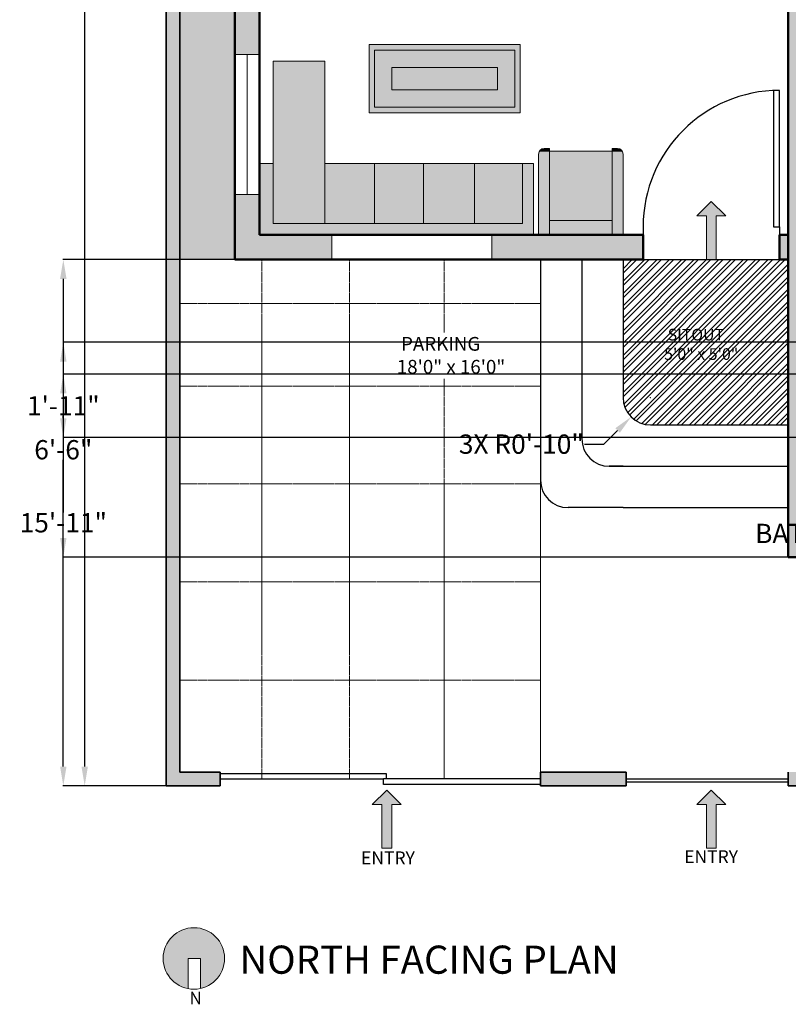
# Model space of a CAD drawing. Units: inches. Extents: x 319 to 870, y 210 to 995.
# Tile 1 of 6: x 319 to 598, y 245 to 603. Entities that reach past the tile are written whole.
import ezdxf

# ---------------------------------------------------------------- set-up
doc = ezdxf.new("R2010")
doc.units = ezdxf.units.IN
doc.header["$MEASUREMENT"] = 0
doc.linetypes.add('DASHED2', pattern=[0.375, 0.25, -0.125])
for name, color, linetype, lineweight in [('A-ANNO-DIMS', 2, 'Continuous', 18), ('A-ANNO-SYMB', 7, 'Continuous', 18), ('A-ANNO-TEXT', 7, 'Continuous', 18), ('A-ANNO-TITL', 7, 'Continuous', 35), ('A-AREA-IDEN', 7, 'Continuous', 18), ('A-DOOR', 4, 'Continuous', 25), ('A-FLOR-PATT', 252, 'Continuous', 13), ('A-FLOR-STRS', 7, 'Continuous', 25), ('A-FURN', 8, 'Continuous', 18), ('A-GLAZ', 4, 'Continuous', 18), ('A-WALL', 7, 'Continuous', 50), ('A-WALL-PATT', 8, 'Continuous', 13), ('C-PROP', 7, 'Continuous', 35), ('C-PROP-PATT', 8, 'Continuous', 13), ('C-PVMT-JNTS', 8, 'DASHED2', 13), ('C-SITE-GATE', 4, 'Continuous', 25)]:
    doc.layers.add(name, color=color, linetype=linetype, lineweight=lineweight)
for name, color, linetype, lineweight, true_color in [('A-ANNO-SYMB-PATT', 16, 'Continuous', 13, 0x6c0707), ('A-FURN-PATT', 30, 'Continuous', 13, 0xf7941d), ('C-SITE-PATT', 126, 'Continuous', 13, 0x1e6f63)]:
    doc.layers.add(name, color=color, linetype=linetype, lineweight=lineweight, true_color=true_color)
doc.styles.get("Standard").update_dxf_attribs({"font": 'arial.ttf'})
doc.dimstyles.get("Standard").update_dxf_attribs({"dimtxt": 7, "dimasz": 7, "dimexe": 0.18, "dimexo": 0.0625, "dimgap": 0.09, "dimtad": 0, "dimtih": 1, "dimtoh": 1, "dimdec": 0, "dimzin": 0, "dimdsep": 46, "dimlunit": 3, "dimtxsty": 'Standard', "dimcen": 0.09, "dimadec": 0, "dimazin": 0, "dimtfac": 1, "dimtdec": 0, "dimtofl": 0, "dimtmove": 0, "dimatfit": 3, "dimfxl": 1, "dimtolj": 1, "dimtzin": 0, "dimarcsym": 0})

# ---------------------------------------------------------------- blocks, each defined once
blk = doc.blocks.new('*U12')
for p, q in [((0, 0), (0, -6)), ((-40, 0), (-40, -6))]:
    blk.add_line(p, q)
blk.add_lwpolyline([(0, 0), (0, 40), (-1.75, 40), (-1.75, 0)], close=True)
blk.add_arc((0, 0), 40, 90, 180)
blk = doc.blocks.new('Arrows - Metric')
h = blk.add_hatch(color=0)
h.set_gradient(color1=(0, 0, 255), rotation=180, tint=1)
h.paths.add_polyline_path([(0, 0), (-6.35, -6.35), (-6.35, -2.159), (-25.4, -2.159), (-25.4, 2.159), (-6.35, 2.159), (-6.35, 6.35)])
at = {"color": 0}
blk.add_lwpolyline([(0, 0), (-6.35, -6.35), (-6.35, -2.159), (-25.4, -2.159), (-25.4, 2.159), (-6.35, 2.159), (-6.35, 6.35)], close=True, dxfattribs=at)
blk = doc.blocks.new('*D22')
at = {"layer": 'A-ANNO-DIMS', "color": 0, "lineweight": -2, "transparency": 16777216}
for p, q in [((371.62, 948.67), (341.96, 948.67)), ((342.14, 941.67), (342.14, 640.33)), ((342.14, 331.67), (342.14, 633)), ((371.62, 324.67), (341.96, 324.67))]:
    blk.add_line(p, q, dxfattribs=at)
at = {"layer": 'A-ANNO-DIMS', "color": 0, "transparency": 16777216}
for points in [[(340.97, 941.67), (343.31, 941.67), (342.14, 948.67)], [(340.97, 331.67), (343.31, 331.67), (342.14, 324.67)]]:
    blk.add_solid(points, dxfattribs=at)
at = {"layer": 'Defpoints', "color": 0, "transparency": 16777216}
for p in [(371.68, 948.67), (342.14, 324.67), (371.68, 324.67)]:
    blk.add_point(p, dxfattribs=at)
at = {"layer": 'A-ANNO-DIMS', "color": 0, "transparency": 16777216, "insert": (342.14, 636.67), "char_height": 7, "attachment_point": 5}
blk.add_mtext("\\A1;52'", dxfattribs=at)
blk = doc.blocks.new('*D39')
at = {"layer": 'A-ANNO-DIMS', "color": 0, "lineweight": -2, "transparency": 16777216}
for p, q in [((689.21, 416.28), (682.21, 416.28)), ((696.21, 417.72), (696.21, 416.1)), ((706.21, 417.72), (706.21, 416.1)), ((713.21, 416.28), (720.21, 416.28))]:
    blk.add_line(p, q, dxfattribs=at)
at = {"layer": 'A-ANNO-DIMS', "color": 0, "transparency": 16777216}
for points in [[(689.21, 417.45), (689.21, 415.11), (696.21, 416.28)], [(713.21, 417.45), (713.21, 415.11), (706.21, 416.28)]]:
    blk.add_solid(points, dxfattribs=at)
at = {"layer": 'Defpoints', "color": 0, "transparency": 16777216}
for p in [(696.21, 417.78), (696.21, 416.28), (706.21, 417.78)]:
    blk.add_point(p, dxfattribs=at)
at = {"layer": 'A-ANNO-DIMS', "color": 0, "transparency": 16777216, "insert": (632.95, 416.28), "char_height": 7, "attachment_point": 5}
blk.add_mtext('\\A1;BATH TAP 0\'-10" TYP.', dxfattribs=at)
blk = doc.blocks.new('*D52')
at = {"layer": 'A-ANNO-DIMS', "color": 0, "lineweight": -2, "transparency": 16777216}
for p, q in [((396.62, 515.67), (334.2, 515.67)), ((334.38, 508.67), (334.38, 423.83)), ((334.38, 331.67), (334.38, 416.5)), ((371.62, 324.67), (334.2, 324.67))]:
    blk.add_line(p, q, dxfattribs=at)
at = {"layer": 'A-ANNO-DIMS', "color": 0, "transparency": 16777216}
for points in [[(333.21, 508.67), (335.55, 508.67), (334.38, 515.67)], [(333.21, 331.67), (335.55, 331.67), (334.38, 324.67)]]:
    blk.add_solid(points, dxfattribs=at)
at = {"layer": 'Defpoints', "color": 0, "transparency": 16777216}
for p in [(334.38, 515.67), (396.68, 515.67), (371.68, 324.67)]:
    blk.add_point(p, dxfattribs=at)
at = {"layer": 'A-ANNO-DIMS', "color": 0, "transparency": 16777216, "insert": (334.38, 420.17), "char_height": 7, "attachment_point": 5}
blk.add_mtext('\\A1;15\'-11"', dxfattribs=at)
blk = doc.blocks.new('*D54')
at = {"layer": 'A-ANNO-DIMS', "color": 0, "lineweight": -2, "transparency": 16777216}
for p, q in [((606.62, 485.67), (334.2, 485.67)), ((334.38, 478.67), (334.38, 450.33)), ((334.38, 414.67), (334.38, 443)), ((597.62, 407.67), (334.2, 407.67))]:
    blk.add_line(p, q, dxfattribs=at)
at = {"layer": 'A-ANNO-DIMS', "color": 0, "transparency": 16777216}
for points in [[(333.21, 478.67), (335.55, 478.67), (334.38, 485.67)], [(333.21, 414.67), (335.55, 414.67), (334.38, 407.67)]]:
    blk.add_solid(points, dxfattribs=at)
at = {"layer": 'Defpoints', "color": 0, "transparency": 16777216}
for p in [(334.38, 485.67), (606.68, 485.67), (597.68, 407.67)]:
    blk.add_point(p, dxfattribs=at)
at = {"layer": 'A-ANNO-DIMS', "color": 0, "transparency": 16777216, "insert": (334.38, 446.67), "char_height": 7, "attachment_point": 5}
blk.add_mtext('\\A1;6\'-6"', dxfattribs=at)
blk = doc.blocks.new('*D56')
at = {"layer": 'A-ANNO-DIMS', "color": 0, "lineweight": -2, "transparency": 16777216}
for p, q in [((675.62, 474.1), (334.2, 474.1)), ((334.38, 467.1), (334.38, 466.2)), ((334.38, 458.09), (334.38, 458.99)), ((675.62, 451.09), (334.2, 451.09))]:
    blk.add_line(p, q, dxfattribs=at)
at = {"layer": 'A-ANNO-DIMS', "color": 0, "transparency": 16777216}
for points in [[(333.21, 467.1), (335.55, 467.1), (334.38, 474.1)], [(333.21, 458.09), (335.55, 458.09), (334.38, 451.09)]]:
    blk.add_solid(points, dxfattribs=at)
at = {"layer": 'Defpoints', "color": 0, "transparency": 16777216}
for p in [(334.38, 474.1), (675.68, 474.1), (675.68, 451.09)]:
    blk.add_point(p, dxfattribs=at)
at = {"layer": 'A-ANNO-DIMS', "color": 0, "transparency": 16777216, "insert": (334.38, 462.6), "char_height": 7, "attachment_point": 5}
blk.add_mtext('\\A1;1\'-11"', dxfattribs=at)
blk = doc.blocks.new('*D60')
at = {"layer": 'A-ANNO-DIMS', "color": 0, "lineweight": -2, "transparency": 16777216}
for p, q in [((547.59, 465.67), (547.77, 465.67)), ((547.68, 465.58), (547.68, 465.76)), ((530.72, 448.7), (535.66, 453.65)), ((523.72, 448.7), (530.72, 448.7))]:
    blk.add_line(p, q, dxfattribs=at)
at = {"layer": 'A-ANNO-DIMS', "color": 0, "transparency": 16777216}
blk.add_solid([(534.84, 454.47), (536.49, 452.82), (540.61, 458.6)], dxfattribs=at)
at = {"layer": 'Defpoints', "color": 0, "transparency": 16777216}
for p in [(547.68, 465.67), (540.61, 458.6)]:
    blk.add_point(p, dxfattribs=at)
at = {"layer": 'A-ANNO-DIMS', "color": 0, "transparency": 16777216, "insert": (500.73, 448.7), "char_height": 7, "attachment_point": 5}
blk.add_mtext('\\A1;3X R0\'-10"', dxfattribs=at)

msp = doc.modelspace()

# ---------------------------------------------------------------- hatches: boundary and pattern name
at = {"layer": 'A-ANNO-SYMB-PATT'}
h = msp.add_hatch(color=256, dxfattribs=at)
h.dxf.hatch_style = 1
h.paths.add_polyline_path([(379.74, 251.07), (379.74, 262.04), (381.79, 262.04), (384.25, 262.04), (384.25, 251.16, 0.350594), (392.95, 262.04, 1), (370.63, 262.04, 0.361033)])
at = {"layer": 'A-FLOR-PATT'}
h = msp.add_hatch(dxfattribs=at)
h.set_pattern_fill('STEEL', color=256)
h.set_pattern_definition([(45, (0, 0), (-2.245064, 2.245064), []), (45, (0, 1.5875), (-2.245064, 2.245064), [])])
h.paths.add_polyline_path([(544.99, 515.67), (537.68, 515.67), (537.68, 465.67, 0.414214), (547.68, 455.67), (597.68, 455.67), (597.68, 515.67), (594.44, 515.67)])
h.paths.add_polyline_path([(551.29, 476.87), (579.21, 476.87), (579.21, 492.64), (551.29, 492.64)], flags=24)
at = {"layer": 'A-FURN-PATT'}
h = msp.add_hatch(color=256, dxfattribs=at)
h.dxf.hatch_style = 1
h.paths.add_polyline_path([(445.43, 593.7), (445.43, 568.99), (500.31, 568.99), (500.31, 593.7)])
h.paths.add_polyline_path([(498.31, 591.7), (498.31, 570.99), (447.43, 570.99), (447.43, 591.7)], flags=16)
h.paths.add_polyline_path([(453.72, 585.41), (492.02, 585.41), (492.02, 577.28), (453.72, 577.28)], flags=0)
h = msp.add_hatch(color=256, dxfattribs=at)
h.dxf.hatch_style = 1
h.paths.add_polyline_path([(447.43, 570.99), (498.31, 570.99), (498.31, 591.7), (447.43, 591.7)])
h.paths.add_polyline_path([(453.72, 577.28), (453.72, 585.41), (492.02, 585.41), (492.02, 577.28)], flags=16)
h = msp.add_hatch(color=256, dxfattribs=at)
h.dxf.hatch_style = 1
h.paths.add_polyline_path([(410.63, 528.72), (429.34, 528.72), (429.34, 550.54), (429.34, 587.64), (410.63, 587.64)])
h = msp.add_hatch(color=256, dxfattribs=at)
h.dxf.hatch_style = 1
h.paths.add_polyline_path([(492.02, 577.28), (492.02, 585.41), (453.72, 585.41), (453.72, 577.28)])
h = msp.add_hatch(color=256, dxfattribs=at)
h.dxf.hatch_style = 1
h.paths.add_polyline_path([(507, 524.67), (511, 524.67), (511, 554.97), (507.27, 554.97, 0.131652), (507, 553.97)])
h = msp.add_hatch(color=256, dxfattribs=at)
h.dxf.hatch_style = 1
h.paths.add_polyline_path([(509, 555.97, 0.267949), (507.27, 554.97), (511, 554.97), (511, 555.97)])
h = msp.add_hatch(color=256, dxfattribs=at)
h.dxf.hatch_style = 1
h.paths.add_polyline_path([(511, 529.89), (533.68, 529.89), (533.68, 554.97), (511, 554.97)])
h = msp.add_hatch(color=256, dxfattribs=at)
h.dxf.hatch_style = 1
h.paths.add_polyline_path([(537.42, 554.97, 0.267949), (535.68, 555.97), (533.68, 555.97), (533.68, 554.97)])
h = msp.add_hatch(color=256, dxfattribs=at)
h.dxf.hatch_style = 1
h.paths.add_polyline_path([(533.68, 524.67), (537.68, 524.67), (537.68, 553.97, 0.131652), (537.42, 554.97), (533.68, 554.97)])
h = msp.add_hatch(color=256, dxfattribs=at)
h.dxf.hatch_style = 1
h.paths.add_polyline_path([(505.09, 524.67), (505.09, 550.54), (501.09, 550.54), (501.09, 528.72), (410.63, 528.72), (410.63, 550.54), (405.68, 550.54), (405.68, 524.67)])
h = msp.add_hatch(color=256, dxfattribs=at)
h.dxf.hatch_style = 1
h.paths.add_polyline_path([(447.34, 528.72), (447.34, 550.54), (429.34, 550.54), (429.34, 528.72)])
h = msp.add_hatch(color=256, dxfattribs=at)
h.dxf.hatch_style = 1
h.paths.add_polyline_path([(447.34, 528.72), (465.15, 528.72), (465.15, 550.54), (447.34, 550.54)])
h = msp.add_hatch(color=256, dxfattribs=at)
h.dxf.hatch_style = 1
h.paths.add_polyline_path([(465.15, 528.72), (483.71, 528.72), (483.71, 550.54), (465.15, 550.54)])
h = msp.add_hatch(color=256, dxfattribs=at)
h.dxf.hatch_style = 1
h.paths.add_polyline_path([(483.71, 528.72), (501.09, 528.72), (501.09, 550.54), (483.71, 550.54)])
h = msp.add_hatch(color=256, dxfattribs=at)
h.dxf.hatch_style = 1
h.paths.add_polyline_path([(533.68, 524.67), (533.68, 529.89), (511, 529.89), (511, 524.67)])
at = {"layer": 'A-WALL-PATT'}
h = msp.add_hatch(color=256, dxfattribs=at)
h.dxf.hatch_style = 1
h.paths.add_polyline_path([(396.68, 590.1), (405.68, 590.1), (405.68, 639.21), (396.68, 639.21)])
h = msp.add_hatch(color=256, dxfattribs=at)
h.dxf.hatch_style = 1
h.paths.add_polyline_path([(606.68, 476.67), (628.53, 476.67), (628.53, 485.67), (606.68, 485.67), (606.68, 614.99), (597.68, 614.99), (597.68, 407.67), (757.68, 407.67), (757.68, 385.48), (766.68, 385.48), (766.68, 431.25), (757.68, 431.25), (757.68, 416.67), (606.68, 416.67)])
h = msp.add_hatch(color=256, dxfattribs=at)
h.dxf.hatch_style = 1
h.paths.add_polyline_path([(431.9, 515.67), (431.9, 524.67), (405.68, 524.67), (405.68, 539.26), (396.68, 539.26), (396.68, 515.67)])
h = msp.add_hatch(color=256, dxfattribs=at)
h.dxf.hatch_style = 1
h.paths.add_polyline_path([(537.68, 515.67), (544.99, 515.67), (544.99, 524.67), (537.68, 524.67), (489.98, 524.67), (489.98, 515.67)])
h = msp.add_hatch(color=256, dxfattribs=at)
h.dxf.hatch_style = 1
h.paths.add_polyline_path([(597.68, 524.67), (594.44, 524.67), (594.44, 515.67), (597.68, 515.67)])
at = {"layer": 'C-PROP-PATT'}
h = msp.add_hatch(color=256, dxfattribs=at)
h.dxf.hatch_style = 1
h.paths.add_polyline_path([(371.68, 324.67), (391.35, 324.67), (391.35, 329.67), (376.68, 329.67), (376.68, 948.67), (371.68, 948.67)])
h = msp.add_hatch(color=256, dxfattribs=at)
h.dxf.hatch_style = 1
h.paths.add_polyline_path([(757.68, 329.67), (597.68, 329.67), (597.68, 324.67), (791.68, 324.67), (791.68, 948.67), (376.68, 948.67), (376.68, 943.67), (786.68, 943.67), (786.68, 329.67), (766.68, 329.67), (766.68, 354.04), (757.68, 354.04)])
h = msp.add_hatch(color=256, dxfattribs=at)
h.dxf.hatch_style = 1
h.paths.add_polyline_path([(538.83, 324.67), (538.83, 329.67), (507.68, 329.67), (507.68, 324.67)])
at = {"layer": 'C-SITE-PATT'}
h = msp.add_hatch(color=256, dxfattribs=at)
h.dxf.hatch_style = 1
h.paths.add_polyline_path([(376.68, 515.67), (396.68, 515.67), (396.68, 923.67), (528.68, 923.67), (606.68, 923.67), (766.68, 923.67), (766.68, 329.67), (786.68, 329.67), (786.68, 943.67), (376.68, 943.67)])
h.paths.add_polyline_path([(392.17, 638.98), (392.17, 682.3), (381.61, 682.3), (381.61, 638.98)], flags=24)
h.paths.add_polyline_path([(772.77, 716.95), (772.77, 673.64), (783.33, 673.64), (783.33, 716.95)], flags=24)
h.paths.add_polyline_path([(542.27, 929.56), (581.61, 929.56), (581.61, 939.15), (542.27, 939.15)], flags=24)

# ---------------------------------------------------------------- linework, layer by layer
at = {"layer": 'A-ANNO-SYMB'}
for p, q in [((381.79, 262.04), (379.74, 262.04)), ((379.74, 262.04), (379.74, 251.07)), ((381.79, 262.04), (384.25, 262.04)), ((384.25, 262.04), (384.25, 251.16))]:
    msp.add_line(p, q, dxfattribs=at)
msp.add_circle((381.79, 262.04), 11.16, dxfattribs=at)
at = {"layer": 'A-DOOR'}
msp.add_line((544.99, 515.67), (594.44, 515.67), dxfattribs=at)
at = {"layer": 'A-FLOR-STRS'}
for p, q in [((507.68, 515.67), (507.68, 455.67)), ((522.68, 515.67), (522.68, 455.67)), ((537.68, 515.67), (537.68, 465.67)), ((507.68, 455.67), (507.68, 435.67)), ((522.68, 455.67), (522.68, 450.67)), ((547.68, 455.67), (597.68, 455.67)), ((532.68, 440.67), (597.68, 440.67)), ((537.68, 440.67), (532.68, 440.67)), ((537.68, 425.67), (517.68, 425.67)), ((537.68, 425.67), (597.68, 425.67))]:
    msp.add_line(p, q, dxfattribs=at)
for centre in [(547.68, 465.67), (532.68, 450.67), (517.68, 435.67)]:
    msp.add_arc(centre, 10, 180, 270, dxfattribs=at)
at = {"layer": 'A-FURN'}
for p, q in [((429.34, 587.64), (410.63, 587.64)), ((410.63, 587.64), (410.63, 528.72)), ((429.34, 550.54), (429.34, 587.64)), ((507, 553.97), (507, 524.67)), ((537.42, 554.97), (507.27, 554.97)), ((511, 555.97), (509, 555.97)), ((511, 555.97), (511, 524.67)), ((535.68, 555.97), (533.68, 555.97)), ((533.68, 524.67), (533.68, 555.97)), ((537.68, 524.67), (537.68, 553.97)), ((410.63, 550.54), (405.68, 550.54)), ((505.09, 550.54), (429.34, 550.54)), ((429.34, 528.72), (429.34, 550.54)), ((447.34, 528.72), (447.34, 550.54)), ((465.15, 528.72), (465.15, 550.54)), ((483.71, 528.72), (483.71, 550.54)), ((501.09, 528.72), (501.09, 550.54)), ((505.09, 524.67), (505.09, 550.54)), ((511, 529.89), (533.68, 529.89)), ((410.63, 528.72), (501.09, 528.72))]:
    msp.add_line(p, q, dxfattribs=at)
for points in [[(445.43, 593.7), (500.31, 593.7), (500.31, 568.99), (445.43, 568.99)], [(447.43, 591.7), (498.31, 591.7), (498.31, 570.99), (447.43, 570.99)], [(453.72, 585.41), (492.02, 585.41), (492.02, 577.28), (453.72, 577.28)]]:
    msp.add_lwpolyline(points, close=True, dxfattribs=at)
for centre, start, end in [((509, 553.97), 90, 180), ((535.68, 553.97), 0, 90)]:
    msp.add_arc(centre, 2, start, end, dxfattribs=at)
at = {"layer": 'A-GLAZ'}
for p, q in [((405.68, 590.1), (396.68, 590.1)), ((401.18, 539.26), (401.18, 590.1)), ((405.68, 539.26), (396.68, 539.26)), ((431.9, 524.67), (431.9, 515.67)), ((489.98, 524.67), (489.98, 515.67))]:
    msp.add_line(p, q, dxfattribs=at)
at = {"layer": 'A-WALL'}
for p, q in [((396.68, 923.67), (396.68, 515.67)), ((405.68, 716.67), (405.68, 524.67)), ((597.68, 614.99), (597.68, 407.67)), ((537.68, 524.67), (405.68, 524.67)), ((544.99, 524.67), (537.68, 524.67)), ((544.99, 515.67), (544.99, 524.67)), ((597.68, 524.67), (594.44, 524.67)), ((594.44, 524.67), (594.44, 515.67)), ((537.68, 515.67), (396.68, 515.67)), ((537.68, 515.67), (537.68, 515.67)), ((537.68, 515.67), (544.99, 515.67)), ((594.44, 515.67), (597.68, 515.67)), ((757.68, 407.67), (597.68, 407.67))]:
    msp.add_line(p, q, dxfattribs=at)
at = {"layer": 'C-PROP'}
for p, q in [((371.68, 948.67), (371.68, 324.67)), ((376.68, 948.67), (376.68, 329.67)), ((376.68, 329.67), (391.35, 329.67)), ((391.35, 329.67), (391.35, 324.67)), ((507.68, 329.67), (507.68, 324.67)), ((507.68, 329.67), (538.83, 329.67)), ((538.83, 329.67), (538.83, 324.67)), ((597.68, 329.67), (597.68, 324.67)), ((371.68, 324.67), (391.35, 324.67)), ((507.68, 324.67), (538.83, 324.67)), ((597.68, 324.67), (791.68, 324.67))]:
    msp.add_line(p, q, dxfattribs=at)
at = {"layer": 'C-PVMT-JNTS'}
for p, q in [((396.68, 515.67), (376.68, 515.67)), ((406.45, 515.67), (406.45, 327.17)), ((438.27, 515.67), (438.27, 327.17)), ((472.72, 515.67), (472.72, 489.26)), ((376.68, 499.77), (507.68, 499.77)), ((472.72, 472.42), (472.72, 327.17)), ((376.68, 469.79), (507.68, 469.79)), ((376.68, 434.27), (507.68, 434.27)), ((507.68, 435.67), (507.68, 324.67)), ((376.68, 398.74), (507.68, 398.74)), ((376.68, 363.04), (507.68, 363.04))]:
    msp.add_line(p, q, dxfattribs=at)
at = {"layer": 'C-SITE-GATE'}
for p, q in [((391.35, 329.17), (450.68, 329.17)), ((450.68, 329.17), (451.68, 329.17)), ((451.68, 329.17), (451.68, 327.17)), ((391.35, 327.17), (450.68, 327.17)), ((507.68, 327.17), (450.68, 327.17)), ((450.68, 325.17), (450.68, 327.17)), ((538.83, 327.17), (597.68, 327.17)), ((538.83, 326.17), (597.68, 326.17)), ((507.68, 325.17), (450.68, 325.17))]:
    msp.add_line(p, q, dxfattribs=at)

# ---------------------------------------------------------------- block references
at = {"layer": 'A-ANNO-SYMB', "xscale": 0.8311720094608933, "yscale": 0.8311720094608933, "zscale": 0.8311720094608933, "rotation": 90}
for p in [(569.71, 536.78), (451.85, 323.16), (569.71, 323.16)]:
    msp.add_blockref('Arrows - Metric', p, dxfattribs=at)
at = {"layer": 'A-DOOR', "xscale": 1.236988369888778, "yscale": 1.236988369888778, "zscale": 1.236988369888778}
msp.add_blockref('*U12', (594.44, 527.59), dxfattribs=at)

# ---------------------------------------------------------------- texts
at = {"layer": 'A-ANNO-SYMB', "insert": (380.19, 249.95), "char_height": 4.56, "attachment_point": 1}
msp.add_mtext_dynamic_manual_height_columns('N', width=80.753, gutter_width=22.79, heights=[0], dxfattribs=at)
at = {"layer": 'A-ANNO-TEXT', "char_height": 4.654, "attachment_point": 1}
for insert in [(442.51, 300.88), (559.88, 301.3)]:
    msp.add_mtext_dynamic_manual_height_columns('{ENTRY}', width=60.2718, gutter_width=23.27, heights=[0], dxfattribs=dict(at, insert=insert))
at = {"layer": 'A-ANNO-TITL', "insert": (398.36, 266.7), "char_height": 10.2135, "attachment_point": 1}
msp.add_mtext_dynamic_manual_height_columns('NORTH FACING PLAN', width=180.9336, gutter_width=51.07, heights=[0], dxfattribs=at)
at = {"layer": 'A-AREA-IDEN', "attachment_point": 1}
for s, width, gutter_width, insert, char_height in [(' SITOUT\\P5\'0" x 5\'0"', 54.723, 21.13, (552.59, 490.54), 4.2255), (' PARKING\\P18\'0" x 16\'0"', 64.6693, 24.97, (455.5, 487.59), 4.9935)]:
    msp.add_mtext_dynamic_manual_height_columns(s, width=width, gutter_width=gutter_width, heights=[0], dxfattribs=dict(at, insert=insert, char_height=char_height))

# ---------------------------------------------------------------- dimensions: what is measured, and where the dimension line sits
at = {"layer": 'A-ANNO-DIMS'}
for base, p1, p2, override, picture, middle in [((342.14, 324.67), (371.68, 948.67), (371.68, 324.67), {"dimclrd": 0, "dimclre": 0, "dimclrt": 0}, '*D22', (342.14, 636.67)), ((334.38, 515.67), (371.68, 324.67), (396.68, 515.67), {"dimdec": 1, "dimlfac": 1, "dimrnd": 0, "dimzin": 1, "dimdsep": 46, "dimlunit": 4, "dimfrac": 2}, '*D52', (334.38, 420.17)), ((334.38, 485.67), (597.68, 407.67), (606.68, 485.67), {"dimdec": 1, "dimlfac": 1, "dimrnd": 0, "dimzin": 1, "dimdsep": 46, "dimlunit": 4, "dimfrac": 2}, '*D54', (334.38, 446.67)), ((334.38, 474.1), (675.68, 451.09), (675.68, 474.1), {"dimdec": 1, "dimlfac": 1, "dimrnd": 0, "dimzin": 1, "dimdsep": 46, "dimlunit": 4, "dimfrac": 2}, '*D56', (334.38, 462.6))]:
    dim = msp.add_linear_dim(base=base, p1=p1, p2=p2, angle=90, dimstyle='Standard', override=override, dxfattribs=at)
    dim.commit()
    dim.dimension.update_dxf_attribs({"geometry": picture, "text_midpoint": middle})
dim = msp.add_radius_dim(center=(547.68, 465.67), mpoint=(540.61, 458.6), text='3X <>', dimstyle='Standard', override={"dimdec": 1, "dimlfac": 1, "dimrnd": 0, "dimzin": 1, "dimdsep": 46, "dimlunit": 4, "dimfrac": 2}, dxfattribs=at)
dim.commit()
dim.dimension.update_dxf_attribs({"geometry": '*D60', "text_midpoint": (500.73, 448.7)})
dim = msp.add_linear_dim(base=(696.21, 416.28), p1=(706.21, 417.78), p2=(696.21, 417.78), angle=180, text='BATH TAP <> TYP.', dimstyle='Standard', override={"dimdec": 1, "dimlfac": 1, "dimrnd": 0, "dimzin": 1, "dimdsep": 46, "dimlunit": 4, "dimfrac": 2}, dxfattribs=at)
dim.commit()
dim.dimension.update_dxf_attribs({"geometry": '*D39', "text_midpoint": (632.95, 416.28)})

doc.saveas('drawing.dxf')
